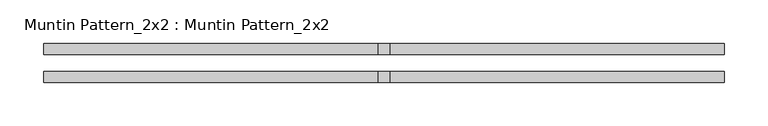
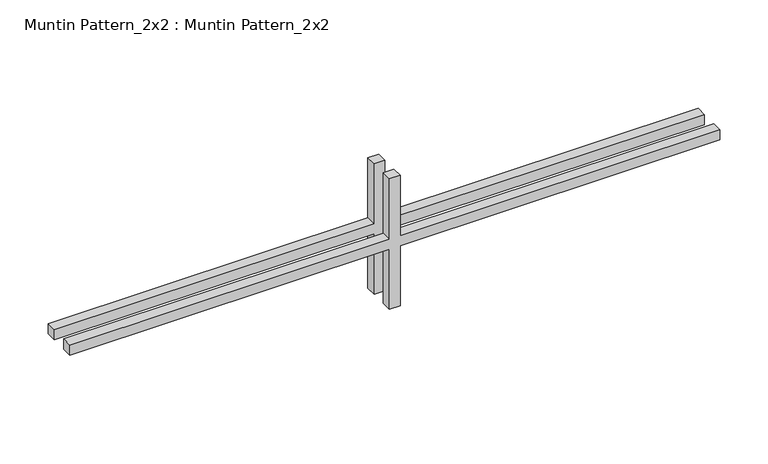
"""IFC4 building model written with IfcOpenShell, lengths in millimetres: proxy geometry, Muntin Pattern_2x2 : Muntin Pattern_2x2."""

from ifc_helpers import new_model, si_unit, frame, origin, place, context, project, spatial, polyline, outline, extrude, source, transform, mapped, element, save


def muntin_pattern_2x2_muntin_pattern_2x2_f17ebf58(model_context):
    return source(origin(), model_context, "Body", "SweptSolid", [
        extrude(outline(polyline([(88.9, -6.35), (88.9, -388.9375), (76.2, -388.9375), (76.2, -6.35), (0.0, -6.35), (0.0, 6.35), (76.2, 6.35), (76.2, 388.9375), (88.9, 388.9375), (88.9, 6.35), (165.1, 6.35), (165.1, -6.35), (88.9, -6.35)])), frame((0.0, -22.225, 0.0), z_axis=(0.0, 1.0, 0.0), x_axis=(0.0, 0.0, 1.0)), (0.0, 0.0, 1.0), 12.7),
        extrude(outline(polyline([(88.9, -6.35), (88.9, -388.9375), (76.2, -388.9375), (76.2, -6.35), (0.0, -6.35), (0.0, 6.35), (76.2, 6.35), (76.2, 388.9375), (88.9, 388.9375), (88.9, 6.35), (165.1, 6.35), (165.1, -6.35), (88.9, -6.35)])), frame((0.0, 9.525, 0.0), z_axis=(0.0, 1.0, 0.0), x_axis=(0.0, 0.0, 1.0)), (0.0, 0.0, 1.0), 12.7),
    ])


if __name__ == "__main__":
    model = new_model("IFC4")
    model_context = context("Model", 3, world=origin())
    ifc_project = project(units=[si_unit("LENGTHUNIT", "METRE", prefix="MILLI")], contexts=[model_context])
    site = spatial("IfcSite", under=ifc_project)
    building = spatial("IfcBuilding", under=site)
    placement = place(None, origin())
    muntin_pattern_2x2_muntin_pattern_2x2_shape = muntin_pattern_2x2_muntin_pattern_2x2_f17ebf58(model_context)
    element("IfcBuildingElementProxy", 1, Name="Muntin Pattern_2x2 : Muntin Pattern_2x2", ObjectType="Muntin Pattern_2x2 : Muntin Pattern_2x2", at=placement, inside=building, context=model_context, shape_type="MappedRepresentation", body=[
        mapped(muntin_pattern_2x2_muntin_pattern_2x2_shape, transform((0.0, 0.0, 0.0), x_axis=(1.0, 0.0, 0.0), y_axis=(0.0, 1.0, 0.0), z_axis=(0.0, 0.0, 1.0))),
    ])
    save(model, "model.ifc")

# Revit data of these elements
# Type "Muntin Pattern_2x2 : Muntin Pattern_2x2"
#   Width [instance default] = 4' - 0"
#   Thickness = 0' - 0 1/2"
#   Height [instance default] = 4' - 0"
#   Distance = 0' - 0 3/4"
#   Interior Material [instance default] = none
#   Exterior Material [instance default] = none
#   Default Elevation = 0
# Element 1 (IfcBuildingElementProxy, "Muntin Pattern_2x2 : Muntin Pattern_2x2")
#   Width = 2' - 6 5/8"
#   Height = 0' - 6 1/2"
#   Interior Material = Wood - Stained
#   Exterior Material = Clad - White
#   Materials on its faces: "Clad - White", "Wood - Stained"
# Materials
#   "Clad - White": class "Wood", colour RGB 242 242 238, transparency 0, Cost = 0
#   "Wood - Stained": class "Wood", colour RGB 224 178 126, transparency 0, Cost = 0
